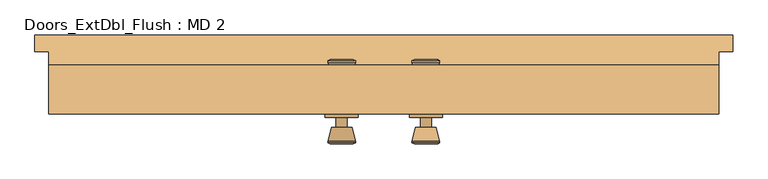
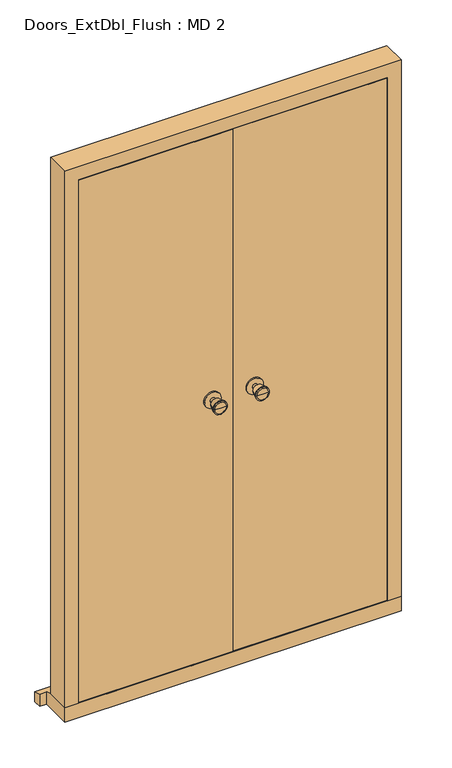
"""IFC4 building model written with IfcOpenShell, lengths in millimetres: door geometry, Doors_ExtDbl_Flush : MD 2."""

from ifc_helpers import new_model, si_unit, point, frame, frame_2d, origin, place, context, project, spatial, polyline, circle_curve, trimmed, segment, composite_curve, outline, extrude, faceted_brep, source, transform, mapped, element, save
from ifc_brep_helpers import plane_surface, cylinder_surface, revolved_surface, advanced_brep


def doors_extdbl_flush_md_2_f65acf09(model_context):
    return source(origin(), model_context, "Body", "SolidModel", [
        advanced_brep(
        [(-76.5, -31.1, 1050.0), (-66.5, -31.1, 1050.0), (-86.5, -31.1, 1050.0), (-96.9758676, -80.1, 1050.0), (-56.0241324, -80.1, 1050.0), (-76.5, -80.1, 1050.0), (-101.5, -78.2721319, 1050.0), (-51.5, -78.2721319, 1050.0), (-101.5, -74.8084537, 1050.0), (-51.5, -74.8084537, 1050.0), (-95.136236, -50.1, 1050.0), (-57.863764, -50.1, 1050.0), (-86.5, -50.1, 1050.0), (-66.5, -50.1, 1050.0)],
        [
            (0, 1),
            (1, 2, circle_curve(frame((-76.5, -31.1, 1050.0), z_axis=(0.0, 1.0, 0.0), x_axis=(1.0, 0.0, 0.0)), 10.0)),
            (2, 0),
            (2, 1, circle_curve(frame((-76.5, -31.1, 1050.0), z_axis=(0.0, 1.0, 0.0), x_axis=(1.0, 0.0, 0.0)), 10.0)),
            (3, 4, circle_curve(frame((-76.5, -80.1, 1050.0), z_axis=(0.0, -1.0, 0.0), x_axis=(1.0, 0.0, 0.0)), 20.4758676)),
            (4, 5),
            (5, 3),
            (4, 3, circle_curve(frame((-76.5, -80.1, 1050.0), z_axis=(0.0, -1.0, 0.0), x_axis=(1.0, 0.0, 0.0)), 20.4758676)),
            (6, 7, circle_curve(frame((-76.5, -78.2721319, 1050.0), z_axis=(0.0, -1.0, 0.0), x_axis=(1.0, 0.0, 0.0)), 25.0)),
            (7, 4),
            (3, 6),
            (7, 6, circle_curve(frame((-76.5, -78.2721319, 1050.0), z_axis=(0.0, -1.0, 0.0), x_axis=(1.0, 0.0, 0.0)), 25.0)),
            (8, 9, circle_curve(frame((-76.5, -74.8084537, 1050.0), z_axis=(0.0, -1.0, 0.0), x_axis=(1.0, 0.0, 0.0)), 25.0)),
            (9, 7),
            (6, 8),
            (9, 8, circle_curve(frame((-76.5, -74.8084537, 1050.0), z_axis=(0.0, -1.0, 0.0), x_axis=(1.0, 0.0, 0.0)), 25.0)),
            (10, 11, circle_curve(frame((-76.5, -50.1, 1050.0), z_axis=(0.0, -1.0, 0.0), x_axis=(1.0, 0.0, 0.0)), 18.636236)),
            (11, 9),
            (8, 10),
            (11, 10, circle_curve(frame((-76.5, -50.1, 1050.0), z_axis=(0.0, -1.0, 0.0), x_axis=(1.0, 0.0, 0.0)), 18.636236)),
            (12, 13, circle_curve(frame((-76.5, -50.1, 1050.0), z_axis=(0.0, -1.0, 0.0), x_axis=(1.0, 0.0, 0.0)), 10.0)),
            (13, 11),
            (10, 12),
            (13, 12, circle_curve(frame((-76.5, -50.1, 1050.0), z_axis=(0.0, -1.0, 0.0), x_axis=(1.0, 0.0, 0.0)), 10.0)),
            (1, 13),
            (12, 2),
        ],
        [
            plane_surface(frame((-76.5, -31.1, 1050.0), z_axis=(0.0, 1.0, 0.0), x_axis=(1.0, 0.0, 0.0))),
            plane_surface(frame((-76.5, -80.1, 1050.0), z_axis=(0.0, -1.0, 0.0), x_axis=(1.0, 0.0, 0.0))),
            revolved_surface(polyline([(-56.0241324, -80.1, 1050.0), (-51.5, -78.2721319, 1050.0)]), (-76.5, -31.1, 1050.0), (0.0, 1.0, 0.0)),
            cylinder_surface(frame((-76.5, -31.1, 1050.0), z_axis=(0.0, 1.0, 0.0), x_axis=(1.0, 0.0, 0.0)), 25.0),
            revolved_surface(polyline([(-51.5, -74.8084537, 1050.0), (-57.863764, -50.1, 1050.0)]), (-76.5, -31.1, 1050.0), (0.0, 1.0, 0.0)),
            plane_surface(frame((-76.5, -50.1, 1050.0), z_axis=(0.0, 1.0, 0.0), x_axis=(1.0, 0.0, 0.0))),
            cylinder_surface(frame((-76.5, -31.1, 1050.0), z_axis=(0.0, 1.0, 0.0), x_axis=(1.0, 0.0, 0.0)), 10.0),
        ],
        [
            (0, [[1, 2, 3]]),
            (0, [[-3, 4, -1]]),
            (1, [[5, 6, 7]]),
            (1, [[8, -7, -6]]),
            (2, [[9, 10, -5, 11]]),
            (2, [[12, -11, -8, -10]]),
            (3, [[13, 14, -9, 15]]),
            (3, [[16, -15, -12, -14]]),
            (4, [[17, 18, -13, 19]]),
            (4, [[20, -19, -16, -18]]),
            (5, [[21, 22, -17, 23]]),
            (5, [[24, -23, -20, -22]]),
            (6, [[-2, 25, -21, 26]]),
            (6, [[-4, -26, -24, -25]]),
        ],
    ),
        extrude(outline(composite_curve([segment(trimmed(circle_curve(frame_2d((1050.0, -76.5)), 30.0), [point((1050.0, -46.5))], [point((1050.0, -106.5))], False, "CARTESIAN"), True, "CONTINUOUS"), segment(trimmed(circle_curve(frame_2d((1050.0, -76.5)), 30.0), [point((1050.0, -106.5))], [point((1050.0, -46.5))], False, "CARTESIAN"), True, "CONTINUOUS")], self_intersect=False)), frame((0.0, -31.1, 0.0), z_axis=(0.0, 1.0, 0.0), x_axis=(0.0, 0.0, 1.0)), (0.0, 0.0, 1.0), 6.0),
        advanced_brep(
        [(-76.5, 24.9, 1050.0), (-86.5, 24.9, 1050.0), (-66.5, 24.9, 1050.0), (-96.9758676, 73.9, 1050.0), (-76.5, 73.9, 1050.0), (-56.0241324, 73.9, 1050.0), (-101.5, 72.0721319, 1050.0), (-51.5, 72.0721319, 1050.0), (-101.5, 68.6084537, 1050.0), (-51.5, 68.6084537, 1050.0), (-95.136236, 43.9, 1050.0), (-57.863764, 43.9, 1050.0), (-86.5, 43.9, 1050.0), (-66.5, 43.9, 1050.0)],
        [
            (0, 1),
            (1, 2, circle_curve(frame((-76.5, 24.9, 1050.0), z_axis=(0.0, -1.0, 0.0), x_axis=(1.0, 0.0, 0.0)), 10.0)),
            (2, 0),
            (2, 1, circle_curve(frame((-76.5, 24.9, 1050.0), z_axis=(0.0, -1.0, 0.0), x_axis=(1.0, 0.0, 0.0)), 10.0)),
            (3, 4),
            (4, 5),
            (5, 3, circle_curve(frame((-76.5, 73.9, 1050.0), z_axis=(0.0, 1.0, 0.0), x_axis=(1.0, 0.0, 0.0)), 20.4758676)),
            (3, 5, circle_curve(frame((-76.5, 73.9, 1050.0), z_axis=(0.0, 1.0, 0.0), x_axis=(1.0, 0.0, 0.0)), 20.4758676)),
            (6, 3),
            (5, 7),
            (7, 6, circle_curve(frame((-76.5, 72.0721319, 1050.0), z_axis=(0.0, 1.0, 0.0), x_axis=(1.0, 0.0, 0.0)), 25.0)),
            (6, 7, circle_curve(frame((-76.5, 72.0721319, 1050.0), z_axis=(0.0, 1.0, 0.0), x_axis=(1.0, 0.0, 0.0)), 25.0)),
            (8, 6),
            (7, 9),
            (9, 8, circle_curve(frame((-76.5, 68.6084537, 1050.0), z_axis=(0.0, 1.0, 0.0), x_axis=(1.0, 0.0, 0.0)), 25.0)),
            (8, 9, circle_curve(frame((-76.5, 68.6084537, 1050.0), z_axis=(0.0, 1.0, 0.0), x_axis=(1.0, 0.0, 0.0)), 25.0)),
            (10, 8),
            (9, 11),
            (11, 10, circle_curve(frame((-76.5, 43.9, 1050.0), z_axis=(0.0, 1.0, 0.0), x_axis=(1.0, 0.0, 0.0)), 18.636236)),
            (10, 11, circle_curve(frame((-76.5, 43.9, 1050.0), z_axis=(0.0, 1.0, 0.0), x_axis=(1.0, 0.0, 0.0)), 18.636236)),
            (12, 10),
            (11, 13),
            (13, 12, circle_curve(frame((-76.5, 43.9, 1050.0), z_axis=(0.0, 1.0, 0.0), x_axis=(1.0, 0.0, 0.0)), 10.0)),
            (12, 13, circle_curve(frame((-76.5, 43.9, 1050.0), z_axis=(0.0, 1.0, 0.0), x_axis=(1.0, 0.0, 0.0)), 10.0)),
            (1, 12),
            (13, 2),
        ],
        [
            plane_surface(frame((-76.5, 24.9, 1050.0), z_axis=(0.0, -1.0, 0.0), x_axis=(1.0, 0.0, 0.0))),
            plane_surface(frame((-76.5, 73.9, 1050.0), z_axis=(0.0, 1.0, 0.0), x_axis=(1.0, 0.0, 0.0))),
            revolved_surface(polyline([(-56.0241324, 73.9, 1050.0), (-51.5, 72.0721319, 1050.0)]), (-76.5, 24.9, 1050.0), (0.0, -1.0, 0.0)),
            cylinder_surface(frame((-76.5, 24.9, 1050.0), z_axis=(0.0, -1.0, 0.0), x_axis=(1.0, 0.0, 0.0)), 25.0),
            revolved_surface(polyline([(-51.5, 68.6084537, 1050.0), (-57.863764, 43.9, 1050.0)]), (-76.5, 24.9, 1050.0), (0.0, -1.0, 0.0)),
            plane_surface(frame((-76.5, 43.9, 1050.0), z_axis=(0.0, -1.0, 0.0), x_axis=(1.0, 0.0, 0.0))),
            cylinder_surface(frame((-76.5, 24.9, 1050.0), z_axis=(0.0, -1.0, 0.0), x_axis=(1.0, 0.0, 0.0)), 10.0),
        ],
        [
            (0, [[1, 2, 3]]),
            (0, [[-3, 4, -1]]),
            (1, [[5, 6, 7]]),
            (1, [[-6, -5, 8]]),
            (2, [[9, -7, 10, 11]]),
            (2, [[-10, -8, -9, 12]]),
            (3, [[13, -11, 14, 15]]),
            (3, [[-14, -12, -13, 16]]),
            (4, [[17, -15, 18, 19]]),
            (4, [[-18, -16, -17, 20]]),
            (5, [[21, -19, 22, 23]]),
            (5, [[-22, -20, -21, 24]]),
            (6, [[25, -23, 26, -2]]),
            (6, [[-26, -24, -25, -4]]),
        ],
    ),
        extrude(outline(composite_curve([segment(trimmed(circle_curve(frame_2d((1050.0, -76.5)), 30.0), [point((1050.0, -46.5))], [point((1050.0, -106.5))], False, "CARTESIAN"), True, "CONTINUOUS"), segment(trimmed(circle_curve(frame_2d((1050.0, -76.5)), 30.0), [point((1050.0, -106.5))], [point((1050.0, -46.5))], False, "CARTESIAN"), True, "CONTINUOUS")], self_intersect=False)), frame((0.0, 18.9, 0.0), z_axis=(0.0, 1.0, 0.0), x_axis=(0.0, 0.0, 1.0)), (0.0, 0.0, 1.0), 6.0),
        advanced_brep(
        [(76.5, -31.1, 1050.0), (86.5, -31.1, 1050.0), (66.5, -31.1, 1050.0), (96.9758676, -80.1, 1050.0), (76.5, -80.1, 1050.0), (56.0241324, -80.1, 1050.0), (101.5, -78.2721319, 1050.0), (51.5, -78.2721319, 1050.0), (101.5, -74.8084537, 1050.0), (51.5, -74.8084537, 1050.0), (95.136236, -50.1, 1050.0), (57.863764, -50.1, 1050.0), (86.5, -50.1, 1050.0), (66.5, -50.1, 1050.0)],
        [
            (0, 1),
            (1, 2, circle_curve(frame((76.5, -31.1, 1050.0), z_axis=(0.0, 1.0, 0.0), x_axis=(-1.0, 0.0, 0.0)), 10.0)),
            (2, 0),
            (2, 1, circle_curve(frame((76.5, -31.1, 1050.0), z_axis=(0.0, 1.0, 0.0), x_axis=(-1.0, 0.0, 0.0)), 10.0)),
            (3, 4),
            (4, 5),
            (5, 3, circle_curve(frame((76.5, -80.1, 1050.0), z_axis=(0.0, -1.0, 0.0), x_axis=(-1.0, 0.0, 0.0)), 20.4758676)),
            (3, 5, circle_curve(frame((76.5, -80.1, 1050.0), z_axis=(0.0, -1.0, 0.0), x_axis=(-1.0, 0.0, 0.0)), 20.4758676)),
            (6, 3),
            (5, 7),
            (7, 6, circle_curve(frame((76.5, -78.2721319, 1050.0), z_axis=(0.0, -1.0, 0.0), x_axis=(-1.0, 0.0, 0.0)), 25.0)),
            (6, 7, circle_curve(frame((76.5, -78.2721319, 1050.0), z_axis=(0.0, -1.0, 0.0), x_axis=(-1.0, 0.0, 0.0)), 25.0)),
            (8, 6),
            (7, 9),
            (9, 8, circle_curve(frame((76.5, -74.8084537, 1050.0), z_axis=(0.0, -1.0, 0.0), x_axis=(-1.0, 0.0, 0.0)), 25.0)),
            (8, 9, circle_curve(frame((76.5, -74.8084537, 1050.0), z_axis=(0.0, -1.0, 0.0), x_axis=(-1.0, 0.0, 0.0)), 25.0)),
            (10, 8),
            (9, 11),
            (11, 10, circle_curve(frame((76.5, -50.1, 1050.0), z_axis=(0.0, -1.0, 0.0), x_axis=(-1.0, 0.0, 0.0)), 18.636236)),
            (10, 11, circle_curve(frame((76.5, -50.1, 1050.0), z_axis=(0.0, -1.0, 0.0), x_axis=(-1.0, 0.0, 0.0)), 18.636236)),
            (12, 10),
            (11, 13),
            (13, 12, circle_curve(frame((76.5, -50.1, 1050.0), z_axis=(0.0, -1.0, 0.0), x_axis=(-1.0, 0.0, 0.0)), 10.0)),
            (12, 13, circle_curve(frame((76.5, -50.1, 1050.0), z_axis=(0.0, -1.0, 0.0), x_axis=(-1.0, 0.0, 0.0)), 10.0)),
            (1, 12),
            (13, 2),
        ],
        [
            plane_surface(frame((76.5, -31.1, 1050.0), z_axis=(0.0, 1.0, 0.0), x_axis=(-1.0, 0.0, 0.0))),
            plane_surface(frame((76.5, -80.1, 1050.0), z_axis=(0.0, -1.0, 0.0), x_axis=(-1.0, 0.0, 0.0))),
            revolved_surface(polyline([(56.0241324, -80.1, 1050.0), (51.5, -78.2721319, 1050.0)]), (76.5, -31.1, 1050.0), (0.0, 1.0, 0.0)),
            cylinder_surface(frame((76.5, -31.1, 1050.0), z_axis=(0.0, 1.0, 0.0), x_axis=(-1.0, 0.0, 0.0)), 25.0),
            revolved_surface(polyline([(51.5, -74.8084537, 1050.0), (57.863764, -50.1, 1050.0)]), (76.5, -31.1, 1050.0), (0.0, 1.0, 0.0)),
            plane_surface(frame((76.5, -50.1, 1050.0), z_axis=(0.0, 1.0, 0.0), x_axis=(-1.0, 0.0, 0.0))),
            cylinder_surface(frame((76.5, -31.1, 1050.0), z_axis=(0.0, 1.0, 0.0), x_axis=(-1.0, 0.0, 0.0)), 10.0),
        ],
        [
            (0, [[1, 2, 3]]),
            (0, [[-3, 4, -1]]),
            (1, [[5, 6, 7]]),
            (1, [[-6, -5, 8]]),
            (2, [[9, -7, 10, 11]]),
            (2, [[-10, -8, -9, 12]]),
            (3, [[13, -11, 14, 15]]),
            (3, [[-14, -12, -13, 16]]),
            (4, [[17, -15, 18, 19]]),
            (4, [[-18, -16, -17, 20]]),
            (5, [[21, -19, 22, 23]]),
            (5, [[-22, -20, -21, 24]]),
            (6, [[25, -23, 26, -2]]),
            (6, [[-26, -24, -25, -4]]),
        ],
    ),
        extrude(outline(composite_curve([segment(trimmed(circle_curve(frame_2d((1050.0, 76.5)), 30.0), [point((1050.0, 46.5))], [point((1050.0, 106.5))], False, "CARTESIAN"), True, "CONTINUOUS"), segment(trimmed(circle_curve(frame_2d((1050.0, 76.5)), 30.0), [point((1050.0, 106.5))], [point((1050.0, 46.5))], False, "CARTESIAN"), True, "CONTINUOUS")], self_intersect=False)), frame((0.0, -31.1, 0.0), z_axis=(0.0, 1.0, 0.0), x_axis=(0.0, 0.0, 1.0)), (0.0, 0.0, 1.0), 6.0),
        advanced_brep(
        [(76.5, 24.9, 1050.0), (66.5, 24.9, 1050.0), (86.5, 24.9, 1050.0), (96.9758676, 73.9, 1050.0), (56.0241324, 73.9, 1050.0), (76.5, 73.9, 1050.0), (101.5, 72.0721319, 1050.0), (51.5, 72.0721319, 1050.0), (101.5, 68.6084537, 1050.0), (51.5, 68.6084537, 1050.0), (95.136236, 43.9, 1050.0), (57.863764, 43.9, 1050.0), (86.5, 43.9, 1050.0), (66.5, 43.9, 1050.0)],
        [
            (0, 1),
            (1, 2, circle_curve(frame((76.5, 24.9, 1050.0), z_axis=(0.0, -1.0, 0.0), x_axis=(-1.0, 0.0, 0.0)), 10.0)),
            (2, 0),
            (2, 1, circle_curve(frame((76.5, 24.9, 1050.0), z_axis=(0.0, -1.0, 0.0), x_axis=(-1.0, 0.0, 0.0)), 10.0)),
            (3, 4, circle_curve(frame((76.5, 73.9, 1050.0), z_axis=(0.0, 1.0, 0.0), x_axis=(-1.0, 0.0, 0.0)), 20.4758676)),
            (4, 5),
            (5, 3),
            (4, 3, circle_curve(frame((76.5, 73.9, 1050.0), z_axis=(0.0, 1.0, 0.0), x_axis=(-1.0, 0.0, 0.0)), 20.4758676)),
            (6, 7, circle_curve(frame((76.5, 72.0721319, 1050.0), z_axis=(0.0, 1.0, 0.0), x_axis=(-1.0, 0.0, 0.0)), 25.0)),
            (7, 4),
            (3, 6),
            (7, 6, circle_curve(frame((76.5, 72.0721319, 1050.0), z_axis=(0.0, 1.0, 0.0), x_axis=(-1.0, 0.0, 0.0)), 25.0)),
            (8, 9, circle_curve(frame((76.5, 68.6084537, 1050.0), z_axis=(0.0, 1.0, 0.0), x_axis=(-1.0, 0.0, 0.0)), 25.0)),
            (9, 7),
            (6, 8),
            (9, 8, circle_curve(frame((76.5, 68.6084537, 1050.0), z_axis=(0.0, 1.0, 0.0), x_axis=(-1.0, 0.0, 0.0)), 25.0)),
            (10, 11, circle_curve(frame((76.5, 43.9, 1050.0), z_axis=(0.0, 1.0, 0.0), x_axis=(-1.0, 0.0, 0.0)), 18.636236)),
            (11, 9),
            (8, 10),
            (11, 10, circle_curve(frame((76.5, 43.9, 1050.0), z_axis=(0.0, 1.0, 0.0), x_axis=(-1.0, 0.0, 0.0)), 18.636236)),
            (12, 13, circle_curve(frame((76.5, 43.9, 1050.0), z_axis=(0.0, 1.0, 0.0), x_axis=(-1.0, 0.0, 0.0)), 10.0)),
            (13, 11),
            (10, 12),
            (13, 12, circle_curve(frame((76.5, 43.9, 1050.0), z_axis=(0.0, 1.0, 0.0), x_axis=(-1.0, 0.0, 0.0)), 10.0)),
            (1, 13),
            (12, 2),
        ],
        [
            plane_surface(frame((76.5, 24.9, 1050.0), z_axis=(0.0, -1.0, 0.0), x_axis=(-1.0, 0.0, 0.0))),
            plane_surface(frame((76.5, 73.9, 1050.0), z_axis=(0.0, 1.0, 0.0), x_axis=(-1.0, 0.0, 0.0))),
            revolved_surface(polyline([(56.0241324, 73.9, 1050.0), (51.5, 72.0721319, 1050.0)]), (76.5, 24.9, 1050.0), (0.0, -1.0, 0.0)),
            cylinder_surface(frame((76.5, 24.9, 1050.0), z_axis=(0.0, -1.0, 0.0), x_axis=(-1.0, 0.0, 0.0)), 25.0),
            revolved_surface(polyline([(51.5, 68.6084537, 1050.0), (57.863764, 43.9, 1050.0)]), (76.5, 24.9, 1050.0), (0.0, -1.0, 0.0)),
            plane_surface(frame((76.5, 43.9, 1050.0), z_axis=(0.0, -1.0, 0.0), x_axis=(-1.0, 0.0, 0.0))),
            cylinder_surface(frame((76.5, 24.9, 1050.0), z_axis=(0.0, -1.0, 0.0), x_axis=(-1.0, 0.0, 0.0)), 10.0),
        ],
        [
            (0, [[1, 2, 3]]),
            (0, [[-3, 4, -1]]),
            (1, [[5, 6, 7]]),
            (1, [[8, -7, -6]]),
            (2, [[9, 10, -5, 11]]),
            (2, [[12, -11, -8, -10]]),
            (3, [[13, 14, -9, 15]]),
            (3, [[16, -15, -12, -14]]),
            (4, [[17, 18, -13, 19]]),
            (4, [[20, -19, -16, -18]]),
            (5, [[21, 22, -17, 23]]),
            (5, [[24, -23, -20, -22]]),
            (6, [[-2, 25, -21, 26]]),
            (6, [[-4, -26, -24, -25]]),
        ],
    ),
        extrude(outline(composite_curve([segment(trimmed(circle_curve(frame_2d((1050.0, 76.5)), 30.0), [point((1050.0, 46.5))], [point((1050.0, 106.5))], False, "CARTESIAN"), True, "CONTINUOUS"), segment(trimmed(circle_curve(frame_2d((1050.0, 76.5)), 30.0), [point((1050.0, 106.5))], [point((1050.0, 46.5))], False, "CARTESIAN"), True, "CONTINUOUS")], self_intersect=False)), frame((0.0, 18.9, 0.0), z_axis=(0.0, 1.0, 0.0), x_axis=(0.0, 0.0, 1.0)), (0.0, 0.0, 1.0), 6.0),
        faceted_brep([(539.1, 63.9, 54.5), (609.6, 63.9, 54.5), (609.6, -25.1, 54.5), (561.1, -25.1, 54.5), (561.1, 21.9, 54.5), (539.1, 21.9, 54.5), (539.1, 63.9, 2039.5), (-539.1, 63.9, 2039.5), (-539.1, 63.9, 54.5), (-609.6, 63.9, 54.5), (-609.6, 63.9, 2110.0), (609.6, 63.9, 2110.0), (609.6, -25.1, 2110.0), (-609.6, -25.1, 2110.0), (-609.6, -25.1, 54.5), (-561.1, -25.1, 54.5), (-561.1, -25.1, 2061.5), (561.1, -25.1, 2061.5), (561.1, 21.9, 2061.5), (-561.1, 21.9, 2061.5), (-561.1, 21.9, 54.5), (-539.1, 21.9, 54.5), (-539.1, 21.9, 2039.5), (539.1, 21.9, 2039.5)], [[[0, 1, 2, 3, 4, 5]], [[1, 0, 6, 7, 8, 9, 10, 11]], [[2, 1, 11, 12]], [[3, 2, 12, 13, 14, 15, 16, 17]], [[4, 3, 17, 18]], [[5, 4, 18, 19, 20, 21, 22, 23]], [[0, 5, 23, 6]], [[7, 22, 21, 8]], [[8, 21, 20, 15, 14, 9]], [[13, 10, 9, 14]], [[19, 16, 15, 20]], [[12, 11, 10, 13]], [[18, 17, 16, 19]], [[6, 23, 22, 7]]]),
        faceted_brep([(634.6, 118.9, 0.0), (634.6, 118.9, 38.5947221), (634.6, 88.9, 47.2703282), (634.6, 88.9, 0.0), (-634.6, 118.9, 38.5947221), (-634.6, 118.9, 0.0), (-634.6, 88.9, 0.0), (-634.6, 88.9, 47.2703282), (609.6, 88.9, 0.0), (609.6, -25.1, 0.0), (-609.6, -25.1, 0.0), (-609.6, 88.9, 0.0), (-609.6, 88.9, 47.2703282), (-609.6, 63.9, 54.5), (609.6, 63.9, 54.5), (609.6, 88.9, 47.2703282), (-609.6, -25.1, 54.5), (609.6, -25.1, 54.5)], [[[0, 1, 2, 3]], [[4, 5, 6, 7]], [[5, 0, 3, 8, 9, 10, 11, 6]], [[1, 0, 5, 4]], [[1, 4, 7, 12, 13, 14, 15, 2]], [[13, 16, 17, 14]], [[16, 10, 9, 17]], [[12, 11, 10, 16, 13]], [[11, 12, 7, 6]], [[8, 15, 14, 17, 9]], [[15, 8, 3, 2]]]),
        extrude(outline(polyline([(558.1, -25.1), (1.5, -25.1), (1.5, 18.9), (558.1, 18.9), (558.1, -25.1)])), frame((0.0, 0.0, 58.5), z_axis=(0.0, 0.0, 1.0), x_axis=(1.0, 0.0, 0.0)), (0.0, 0.0, 1.0), 2000.0),
        extrude(outline(polyline([(-1.5, -25.1), (-558.1, -25.1), (-558.1, 18.9), (-1.5, 18.9), (-1.5, -25.1)])), frame((0.0, 0.0, 58.5), z_axis=(0.0, 0.0, 1.0), x_axis=(1.0, 0.0, 0.0)), (0.0, 0.0, 1.0), 2000.0),
    ])


if __name__ == "__main__":
    model = new_model("IFC4")
    model_context = context("Model", 3, world=origin())
    ifc_project = project(units=[si_unit("LENGTHUNIT", "METRE", prefix="MILLI")], contexts=[model_context])
    site = spatial("IfcSite", under=ifc_project)
    building = spatial("IfcBuilding", under=site)
    placement = place(None, origin())
    doors_extdbl_flush_md_2_shape = doors_extdbl_flush_md_2_f65acf09(model_context)
    element("IfcDoor", 1, ObjectType="Doors_ExtDbl_Flush : MD 2", at=placement, inside=building, context=model_context, shape_type="MappedRepresentation", body=[
        mapped(doors_extdbl_flush_md_2_shape, transform((0.0, 0.0, 0.0), x_axis=(1.0, 0.0, 0.0), y_axis=(0.0, 1.0, 0.0), z_axis=(0.0, 0.0, 1.0))),
    ])
    save(model, "model.ifc")

# Revit data of these elements
# Type "Doors_ExtDbl_Flush : MD 2"
#   Type Mark = "51"
#   Type Comments = "External Double"
#   Operation = "DoubleDoorSingleSwing"
#   Keynote = "L20"
#   Analytic Construction = "Metal"
#   Wrap Layers (Ext) from Ext = 0' - 4.03543"
#   Wrap Layers (Int) from Ext = 0' - 6.98819"
#   Thickness = 0' - 1.73228"
#   Rough Width = 4' - 0"
#   Rough Height = 6' - 11.07087"
#   O/A Frame Width = 0' - 2.51969"
#   Heat Transfer Coefficient (U) = 3.7021 W/(m²·K)
#   Handle Z Distance = 3' - 5.33858"
#   FrameWidth = 0' - 1.65354"
#   FrameOffset - External = 0' - 0.98425"
#   FrameDepth = 0' - 3.50394"
#   Door Panel Width = 1' - 9.91339"
#   Door Panel Thickness = 0' - 1.73228"
#   Door Panel Height = 6' - 6.74016"
#   Cill Thickness = 0' - 2.14567"
#   Cill Projection = 0' - 1.1811"
#   Handle X Distance = 0' - 2.95276"
#   Height = 6' - 11.07087"
#   Structural Tolerance = 0' - 0.25591"
#   Tolerance = 0' - 0.11811"
#   Undercut = 0' - 0.15748"
#   Width = 4' - 0"
#   Cill Extension = 0' - 0.98425"
#   Cavity Closer Width = 0' - 1.9685"
#   Cavity Closer Offset from Ext = 0' - 4.03543"
#   Cavity Closer Depth = 0' - 3.34646"
#   Vis - Ironmongery = yes
#   Vis - Cavity Closers = yes
#   Function = 1
#   Material Door = Door - Panel
#   Material Frame = Door - Frame/Mullion
#   Material Ironmongery = Door - Handle
#   Visual Light Transmittance = 0
#   Thermal Resistance (R) = 0
#   Solar Heat Gain Coefficient = 0
#   Wall Closure = (empty or 0)
# Element 1 (IfcDoor, "Doors_ExtDbl_Flush : MD 2")
#   Materials on its faces: "Door - Handle", "Door - Frame/Mullion", "Door - Panel"
# Materials
#   "Door - Panel": class "Wood", colour RGB 210 159 95, transparency 0, Keynote = "L20", Cost = 0
#   "Door - Frame/Mullion": class "Wood", colour RGB 212 179 113, transparency 0, Keynote = "L20", Cost = 0
#   "Door - Handle": colour RGB 0 0 0, transparency 0, Keynote = "P21", Cost = 0
